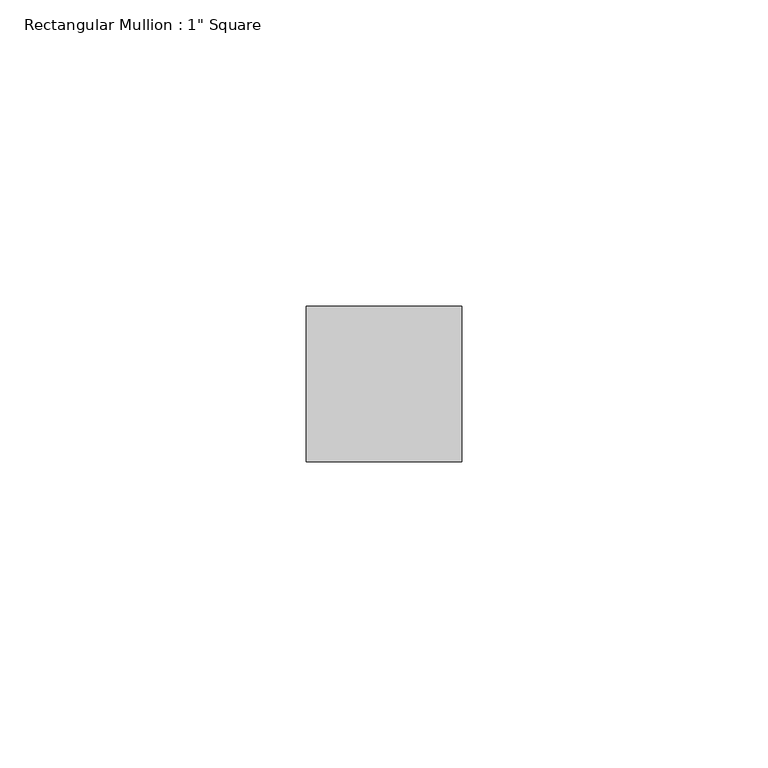
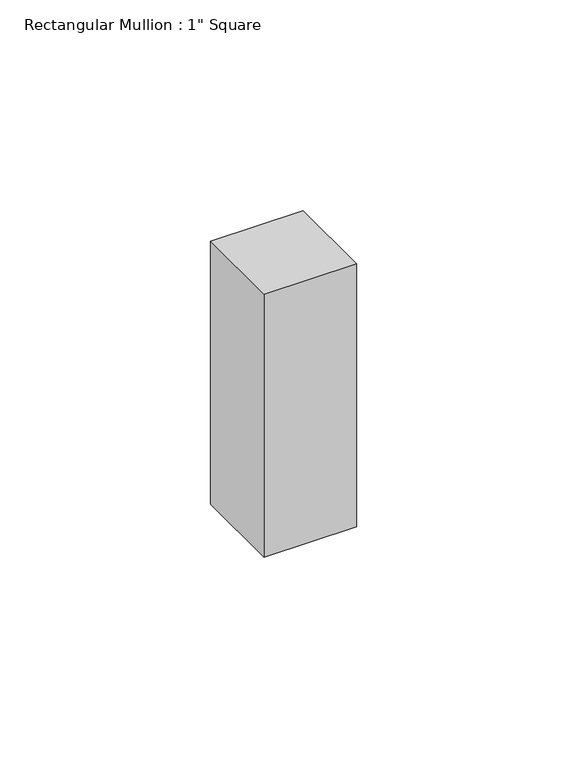
"""IFC4 building model written with IfcOpenShell, lengths in millimetres: member geometry."""

from ifc_helpers import new_model, si_unit, frame, origin, place, context, project, spatial, polyline, outline, extrude, source, transform, mapped, element, save


def member_838ad8ec(model_context):
    return source(origin(), model_context, "Body", "SweptSolid", [
        extrude(outline(polyline([(0.0, 12.7), (0.0, -12.7), (-25.4, -12.7), (-25.4, 12.7), (0.0, 12.7)])), frame((0.0, 0.0, -76.2), z_axis=(0.0, 0.0, 1.0), x_axis=(1.0, 0.0, 0.0)), (0.0, 0.0, 1.0), 76.2),
    ])


if __name__ == "__main__":
    model = new_model("IFC4")
    model_context = context("Model", 3, world=origin())
    ifc_project = project(units=[si_unit("LENGTHUNIT", "METRE", prefix="MILLI")], contexts=[model_context])
    site = spatial("IfcSite", under=ifc_project)
    building = spatial("IfcBuilding", under=site)
    placement = place(None, origin())
    member_shape = member_838ad8ec(model_context)
    element("IfcMember", 1, ObjectType="Rectangular Mullion : 1\" Square", at=placement, inside=building, context=model_context, shape_type="MappedRepresentation", body=[
        mapped(member_shape, transform((0.0, 0.0, 0.0), x_axis=(1.0, 0.0, 0.0), y_axis=(0.0, 1.0, 0.0), z_axis=(0.0, 0.0, 1.0))),
    ])
    save(model, "model.ifc")

# Revit data of these elements
# Type "Rectangular Mullion : 1\" Square"
#   built-in parameter 1007304 = 0.0833333 (stored number, unit not read)
#   built-in parameter 1007301 = 0.0416667 (stored number, unit not read)
#   built-in parameter 1007300 = 0.0416667 (stored number, unit not read)
# Element 1 (IfcMember, "Rectangular Mullion : 1\" Square")
#   Materials on its faces: "black"
# Materials
#   "black": class "Generic", colour RGB 120 120 120, transparency 0, Cost = 0
